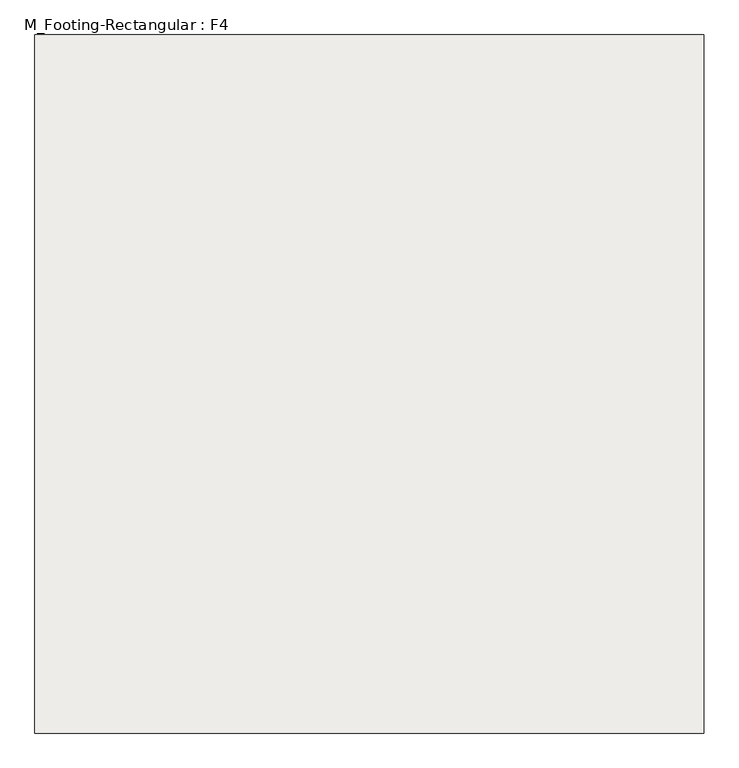
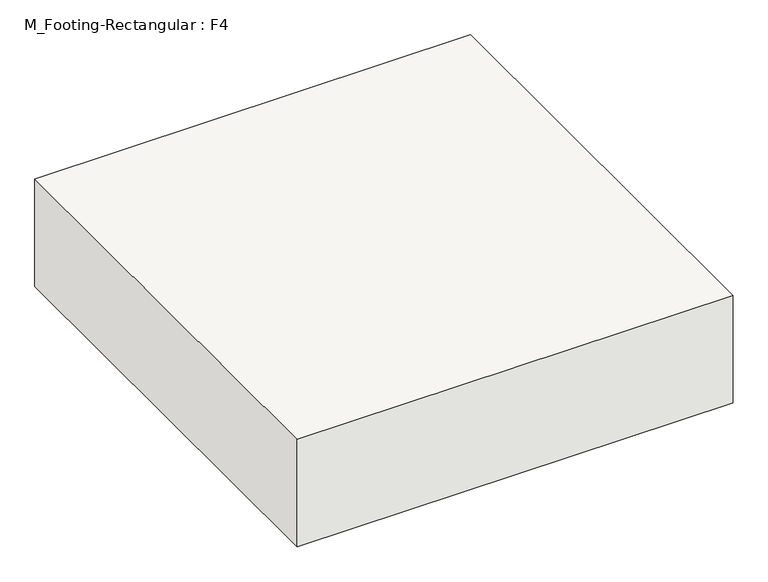
"""IFC4 building model written with IfcOpenShell, lengths in millimetres: slab geometry, M_Footing-Rectangular : F4."""

from ifc_helpers import new_model, si_unit, frame, origin, place, context, project, spatial, polyline, outline, extrude, source, transform, mapped, element, save


def m_footing_rectangular_f4_fcff0cd7(model_context):
    return source(origin(), model_context, "Body", "SweptSolid", [
        extrude(outline(polyline([(876.3, 914.4), (876.3, -914.4), (-876.3, -914.4), (-876.3, 914.4), (876.3, 914.4)])), frame((0.0, 0.0, -457.2), z_axis=(0.0, 0.0, 1.0), x_axis=(1.0, 0.0, 0.0)), (0.0, 0.0, 1.0), 457.2),
    ])


if __name__ == "__main__":
    model = new_model("IFC4")
    model_context = context("Model", 3, world=origin())
    ifc_project = project(units=[si_unit("LENGTHUNIT", "METRE", prefix="MILLI")], contexts=[model_context])
    site = spatial("IfcSite", under=ifc_project)
    building = spatial("IfcBuilding", under=site)
    placement = place(None, origin())
    m_footing_rectangular_f4_shape = m_footing_rectangular_f4_fcff0cd7(model_context)
    element("IfcSlab", 1, ObjectType="M_Footing-Rectangular : F4", at=placement, inside=building, context=model_context, shape_type="MappedRepresentation", body=[
        mapped(m_footing_rectangular_f4_shape, transform((0.0, 0.0, 0.0), x_axis=(1.0, 0.0, 0.0), y_axis=(0.0, 1.0, 0.0), z_axis=(0.0, 0.0, 1.0))),
    ])
    save(model, "model.ifc")

# Revit data of these elements
# Type "M_Footing-Rectangular : F4"
#   Width = 1752.6 mm
#   Length = 1828.8 mm
#   Foundation Thickness = 457.2 mm
#   Structural Material [instance default] = Concrete, Cast-in-Place gray
#   Assembly Code = ""
# Element 1 (IfcSlab, "M_Footing-Rectangular : F4")
#   Materials on its faces: "Concrete, Cast-in-Place gray"
# Materials
#   "Concrete, Cast-in-Place gray": class "Concrete", colour RGB 192 192 192, transparency 0, Description = "Cast-in-place concrete", Cost = 0
